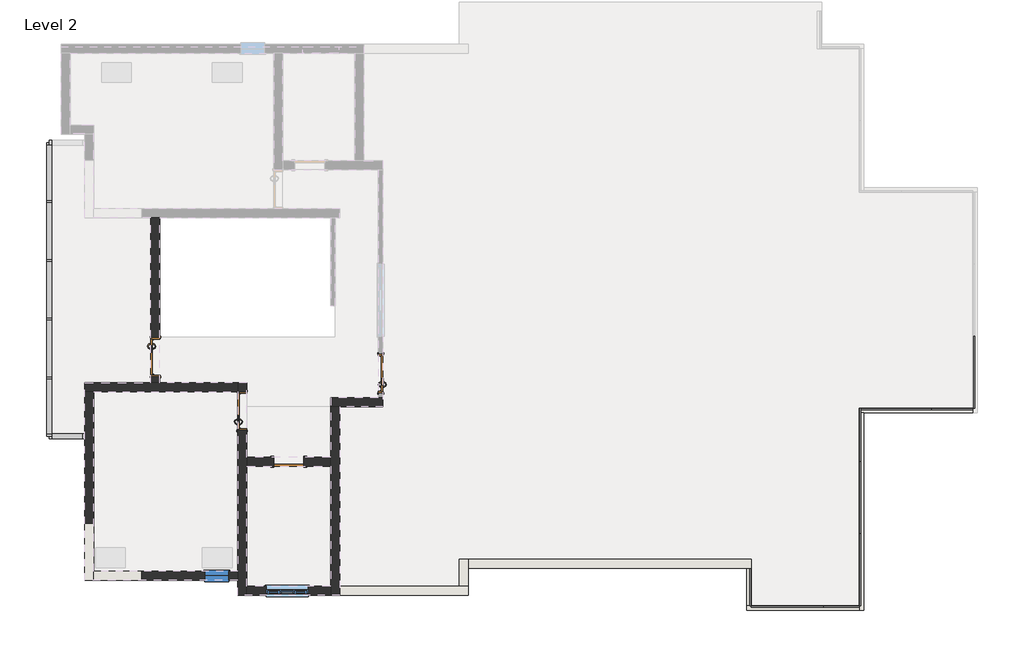
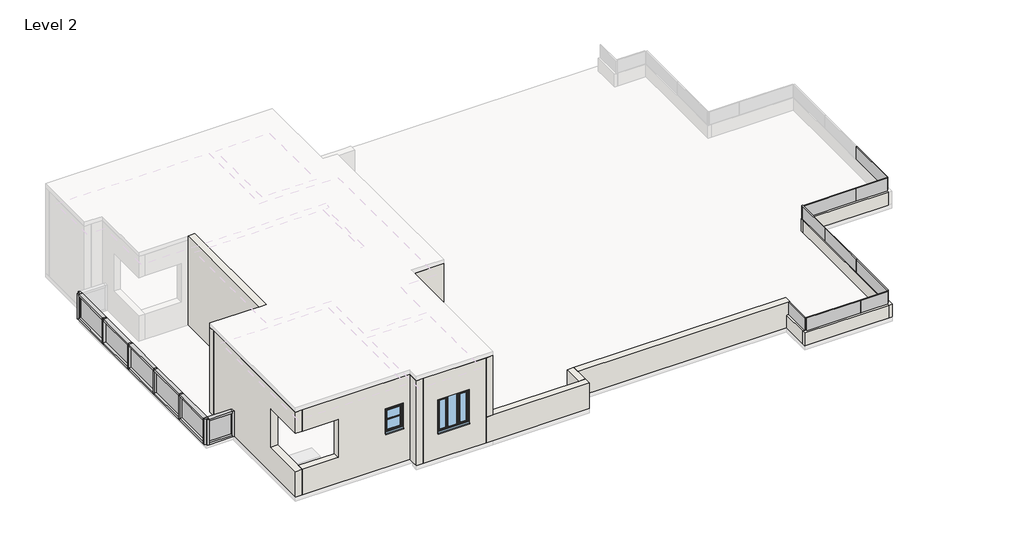
# One storey, part 1 of 2: 21 members, 16 walls, 15 plates, 4 doors, 2 windows.
"""IFC4 building model written with IfcOpenShell, lengths in millimetres."""

from ifc_helpers import new_model, si_unit, frame, origin, place, context, project, spatial, polyline, outline, extrude, faceted_brep, transform, mapped, element, save
from components import door_3dbecc4b, door_cca51ba5, door_181986ca, door_a1484949, member_429f6687, member_c646c215, member_7ec67256, member_73c23c35, member_410c6227, system_panel_glazed_cc3a876e, system_panel_glazed_f05af352, system_panel_glazed_b74e51ee, system_panel_glazed_cfd93610, system_panel_glazed_20ce4246, system_panel_glazed_26639370, system_panel_glazed_ff4fffb2, system_panel_glazed_c2969f63, windows_sgl_swept_head_window_2_x3_cc7253b0, window_63c4cdf6

model = new_model("IFC4")

# Units and contexts
model_context = context("Model", 3, world=origin())
ifc_project = project(units=[si_unit("LENGTHUNIT", "METRE", prefix="MILLI")], contexts=[model_context])

# Site, building, storey
site = spatial("IfcSite", under=ifc_project)
building = spatial("IfcBuilding", under=site)
storey = spatial("IfcBuildingStorey", under=building, Name="Level 2", Elevation=3200.4)

# Doors
placement = place(None, origin())
door_shape = door_3dbecc4b(model_context)
element("IfcDoor", 1, ObjectType="Doors_IntSgl_4 : Internal Door 3'3\"X7'", at=placement, inside=storey, context=model_context, shape_type="MappedRepresentation", body=[
    mapped(door_shape, transform((-3102.7378503, -1463.5864583, 3200.4), x_axis=(0.0, 1.0, 0.0), y_axis=(-1.0, 0.0, 0.0), z_axis=(0.0, 0.0, 1.0))),
])
door_2_shape = door_cca51ba5(model_context)
element("IfcDoor", 2, ObjectType="Doors_IntSgl_4 : Internal Door 3'3\"X7'", at=placement, inside=storey, context=model_context, shape_type="MappedRepresentation", body=[
    mapped(door_2_shape, transform((-5312.0457903, -91.9864583, 3200.4), x_axis=(0.0, -1.0, 0.0), y_axis=(1.0, 0.0, 0.0), z_axis=(0.0, 0.0, 1.0))),
])
door_3_shape = door_181986ca(model_context)
element("IfcDoor", 3, ObjectType="Doors_IntSgl_4 : Internal Door 3'3\"X7'", at=placement, inside=storey, context=model_context, shape_type="MappedRepresentation", body=[
    mapped(door_3_shape, transform((421.5121497, -511.0864583, 3200.4), x_axis=(0.0, 1.0, 0.0), y_axis=(-1.0, 0.0, 0.0), z_axis=(0.0, 0.0, 1.0))),
])
door_4_shape = door_a1484949(model_context)
element("IfcDoor", 4, ObjectType="Single-Flush : 2'6\"", at=placement, inside=storey, context=model_context, shape_type="MappedRepresentation", body=[
    mapped(door_4_shape, transform((-1921.6378503, -2759.0648645, 3200.4), x_axis=(-1.0, 0.0, 0.0), y_axis=(0.0, -1.0, 0.0), z_axis=(0.0, 0.0, 1.0))),
])

# Members
member_shape = member_429f6687(model_context)
element("IfcMember", 5, ObjectType="Rectangular Mullion : 2.5\" x 5\" rectangular", at=placement, inside=storey, context=model_context, shape_type="MappedRepresentation", body=[
    mapped(member_shape, transform((-7166.7378503, -2111.2864583, 4114.8), x_axis=(0.0, 0.0, 1.0), y_axis=(0.0, -1.0, 0.0), z_axis=(1.0, 0.0, 0.0))),
])
element("IfcMember", 6, ObjectType="Rectangular Mullion : 2.5\" x 5\" rectangular", at=placement, inside=storey, context=model_context, shape_type="MappedRepresentation", body=[
    mapped(member_shape, transform((-7954.1378503, -2111.2864583, 3200.4), x_axis=(0.0, 0.0, -1.0), y_axis=(0.0, -1.0, 0.0), z_axis=(-1.0, 0.0, 0.0))),
])
member_2_shape = member_c646c215(model_context)
element("IfcMember", 7, ObjectType="Rectangular Mullion : 2.5\" x 5\" rectangular", at=placement, inside=storey, context=model_context, shape_type="MappedRepresentation", body=[
    mapped(member_2_shape, transform((-8017.6378503, -2047.7864583, 4114.8), x_axis=(0.0, 0.0, 1.0), y_axis=(-1.0, 0.0, 0.0), z_axis=(0.0, -1.0, 0.0))),
])
element("IfcMember", 8, ObjectType="Rectangular Mullion : 2.5\" x 5\" rectangular", at=placement, inside=storey, context=model_context, shape_type="MappedRepresentation", body=[
    mapped(member_2_shape, transform((-8017.6378503, 3894.412299, 4114.8), x_axis=(0.0, 0.0, 1.0), y_axis=(-1.0, 0.0, 0.0), z_axis=(0.0, -1.0, 0.0))),
])
member_3_shape = member_7ec67256(model_context)
element("IfcMember", 9, ObjectType="Rectangular Mullion : 2.5\" x 5\" rectangular", at=placement, inside=storey, context=model_context, shape_type="MappedRepresentation", body=[
    mapped(member_3_shape, transform((-8017.6378503, 2400.9251098, 4114.8), x_axis=(0.0, 0.0, 1.0), y_axis=(-1.0, 0.0, 0.0), z_axis=(0.0, -1.0, 0.0))),
])
element("IfcMember", 10, ObjectType="Rectangular Mullion : 2.5\" x 5\" rectangular", at=placement, inside=storey, context=model_context, shape_type="MappedRepresentation", body=[
    mapped(member_3_shape, transform((-8017.6378503, 907.4379205, 4114.8), x_axis=(0.0, 0.0, 1.0), y_axis=(-1.0, 0.0, 0.0), z_axis=(0.0, -1.0, 0.0))),
])
element("IfcMember", 11, ObjectType="Rectangular Mullion : 2.5\" x 5\" rectangular", at=placement, inside=storey, context=model_context, shape_type="MappedRepresentation", body=[
    mapped(member_3_shape, transform((-8017.6378503, -586.0492687, 4114.8), x_axis=(0.0, 0.0, 1.0), y_axis=(-1.0, 0.0, 0.0), z_axis=(0.0, -1.0, 0.0))),
])
element("IfcMember", 12, ObjectType="Rectangular Mullion : 2.5\" x 5\" rectangular", at=placement, inside=storey, context=model_context, shape_type="MappedRepresentation", body=[
    mapped(member_2_shape, transform((-8017.6378503, 5292.6494886, 3200.4), x_axis=(0.0, 0.0, -1.0), y_axis=(-1.0, 0.0, 0.0), z_axis=(0.0, 1.0, 0.0))),
])
element("IfcMember", 13, ObjectType="Rectangular Mullion : 2.5\" x 5\" rectangular", at=placement, inside=storey, context=model_context, shape_type="MappedRepresentation", body=[
    mapped(member_2_shape, transform((-8017.6378503, -649.5492687, 3200.4), x_axis=(0.0, 0.0, -1.0), y_axis=(-1.0, 0.0, 0.0), z_axis=(0.0, 1.0, 0.0))),
])
element("IfcMember", 14, ObjectType="Rectangular Mullion : 2.5\" x 5\" rectangular", at=placement, inside=storey, context=model_context, shape_type="MappedRepresentation", body=[
    mapped(member_3_shape, transform((-8017.6378503, 3830.912299, 3200.4), x_axis=(0.0, 0.0, -1.0), y_axis=(-1.0, 0.0, 0.0), z_axis=(0.0, 1.0, 0.0))),
])
element("IfcMember", 15, ObjectType="Rectangular Mullion : 2.5\" x 5\" rectangular", at=placement, inside=storey, context=model_context, shape_type="MappedRepresentation", body=[
    mapped(member_3_shape, transform((-8017.6378503, 2337.4251098, 3200.4), x_axis=(0.0, 0.0, -1.0), y_axis=(-1.0, 0.0, 0.0), z_axis=(0.0, 1.0, 0.0))),
])
element("IfcMember", 16, ObjectType="Rectangular Mullion : 2.5\" x 5\" rectangular", at=placement, inside=storey, context=model_context, shape_type="MappedRepresentation", body=[
    mapped(member_3_shape, transform((-8017.6378503, 843.9379205, 3200.4), x_axis=(0.0, 0.0, -1.0), y_axis=(-1.0, 0.0, 0.0), z_axis=(0.0, 1.0, 0.0))),
])
member_4_shape = member_73c23c35(model_context)
element("IfcMember", 17, ObjectType="Rectangular Mullion : 2.5\" x 5\" rectangular", at=placement, inside=storey, context=model_context, shape_type="MappedRepresentation", body=[
    mapped(member_4_shape, transform((-8017.6378503, 5356.1494886, 3200.4), x_axis=(-1.0, 0.0, 0.0), y_axis=(0.0, 1.0, 0.0), z_axis=(0.0, 0.0, -1.0))),
])
element("IfcMember", 18, ObjectType="Rectangular Mullion : 2.5\" x 5\" rectangular", at=placement, inside=storey, context=model_context, shape_type="MappedRepresentation", body=[
    mapped(member_4_shape, transform((-8017.6378503, -2111.2864583, 3200.4), x_axis=(0.0, -1.0, 0.0), y_axis=(-1.0, 0.0, 0.0), z_axis=(0.0, 0.0, -1.0))),
])
element("IfcMember", 19, ObjectType="Rectangular Mullion : 2.5\" x 5\" rectangular", at=placement, inside=storey, context=model_context, shape_type="MappedRepresentation", body=[
    mapped(member_4_shape, transform((-7103.2378503, -2111.2864583, 3200.4), x_axis=(1.0, 0.0, 0.0), y_axis=(0.0, -1.0, 0.0), z_axis=(0.0, 0.0, -1.0))),
])
element("IfcMember", 20, ObjectType="Rectangular Mullion : 2.5\" x 5\" rectangular", at=placement, inside=storey, context=model_context, shape_type="MappedRepresentation", body=[
    mapped(member_4_shape, transform((-8017.6378503, 5356.1494886, 4114.8), x_axis=(0.0, 1.0, 0.0), y_axis=(-1.0, 0.0, 0.0), z_axis=(0.0, 0.0, 1.0))),
])
element("IfcMember", 21, ObjectType="Rectangular Mullion : 2.5\" x 5\" rectangular", at=placement, inside=storey, context=model_context, shape_type="MappedRepresentation", body=[
    mapped(member_4_shape, transform((-8017.6378503, -2111.2864583, 4114.8), x_axis=(-1.0, 0.0, 0.0), y_axis=(0.0, -1.0, 0.0), z_axis=(0.0, 0.0, 1.0))),
])
member_5_shape = member_410c6227(model_context)
element("IfcMember", 22, ObjectType="Rectangular Mullion : 2.5\" x 5\" rectangular", at=placement, inside=storey, context=model_context, shape_type="MappedRepresentation", body=[
    mapped(member_5_shape, transform((-8017.6378503, 3862.662299, 3200.4), x_axis=(0.0, -1.0, 0.0), y_axis=(-1.0, 0.0, 0.0), z_axis=(0.0, 0.0, -1.0))),
])
element("IfcMember", 23, ObjectType="Rectangular Mullion : 2.5\" x 5\" rectangular", at=placement, inside=storey, context=model_context, shape_type="MappedRepresentation", body=[
    mapped(member_5_shape, transform((-8017.6378503, 2369.1751098, 3200.4), x_axis=(0.0, -1.0, 0.0), y_axis=(-1.0, 0.0, 0.0), z_axis=(0.0, 0.0, -1.0))),
])
element("IfcMember", 24, ObjectType="Rectangular Mullion : 2.5\" x 5\" rectangular", at=placement, inside=storey, context=model_context, shape_type="MappedRepresentation", body=[
    mapped(member_5_shape, transform((-8017.6378503, 875.6879205, 3200.4), x_axis=(0.0, -1.0, 0.0), y_axis=(-1.0, 0.0, 0.0), z_axis=(0.0, 0.0, -1.0))),
])
element("IfcMember", 25, ObjectType="Rectangular Mullion : 2.5\" x 5\" rectangular", at=placement, inside=storey, context=model_context, shape_type="MappedRepresentation", body=[
    mapped(member_5_shape, transform((-8017.6378503, -617.7992687, 3200.4), x_axis=(0.0, -1.0, 0.0), y_axis=(-1.0, 0.0, 0.0), z_axis=(0.0, 0.0, -1.0))),
])

# Plates
system_panel_glazed_shape = system_panel_glazed_cc3a876e(model_context)
element("IfcPlate", 26, ObjectType="System Panel : Glazed", at=placement, inside=storey, context=model_context, shape_type="MappedRepresentation", body=[
    mapped(system_panel_glazed_shape, transform((9851.2621497, -5940.3364583, 3657.6), x_axis=(0.0, -1.0, 0.0), y_axis=(1.0, 0.0, 0.0), z_axis=(0.0, 0.0, 1.0))),
])
system_panel_glazed_2_shape = system_panel_glazed_f05af352(model_context)
element("IfcPlate", 27, ObjectType="System Panel : Glazed", at=placement, inside=storey, context=model_context, shape_type="MappedRepresentation", body=[
    mapped(system_panel_glazed_2_shape, transform((10765.6621499, -6416.5864583, 3657.6), x_axis=(1.0, 0.0, 0.0), y_axis=(0.0, 1.0, 0.0), z_axis=(0.0, 0.0, 1.0))),
])
element("IfcPlate", 28, ObjectType="System Panel : Glazed", at=placement, inside=storey, context=model_context, shape_type="MappedRepresentation", body=[
    mapped(system_panel_glazed_2_shape, transform((12594.4621497, -5502.1864581, 3657.6), x_axis=(0.0, 1.0, 0.0), y_axis=(-1.0, 0.0, 0.0), z_axis=(0.0, 0.0, 1.0))),
])
element("IfcPlate", 29, ObjectType="System Panel : Glazed", at=placement, inside=storey, context=model_context, shape_type="MappedRepresentation", body=[
    mapped(system_panel_glazed_2_shape, transform((12594.4621497, -3673.386458, 3657.6), x_axis=(0.0, 1.0, 0.0), y_axis=(-1.0, 0.0, 0.0), z_axis=(0.0, 0.0, 1.0))),
])
element("IfcPlate", 30, ObjectType="System Panel : Glazed", at=placement, inside=storey, context=model_context, shape_type="MappedRepresentation", body=[
    mapped(system_panel_glazed_2_shape, transform((13508.8621499, -1387.3864583, 3657.6), x_axis=(1.0, 0.0, 0.0), y_axis=(0.0, 1.0, 0.0), z_axis=(0.0, 0.0, 1.0))),
])
element("IfcPlate", 31, ObjectType="System Panel : Glazed", at=placement, inside=storey, context=model_context, shape_type="MappedRepresentation", body=[
    mapped(system_panel_glazed_2_shape, transform((15490.0621497, -472.9864581, 3657.6), x_axis=(0.0, 1.0, 0.0), y_axis=(-1.0, 0.0, 0.0), z_axis=(0.0, 0.0, 1.0))),
])
system_panel_glazed_3_shape = system_panel_glazed_b74e51ee(model_context)
element("IfcPlate", 32, ObjectType="System Panel : Glazed", at=placement, inside=storey, context=model_context, shape_type="MappedRepresentation", body=[
    mapped(system_panel_glazed_3_shape, transform((12137.2621499, -6416.5864583, 3657.6), x_axis=(1.0, 0.0, 0.0), y_axis=(0.0, 1.0, 0.0), z_axis=(0.0, 0.0, 1.0))),
])
system_panel_glazed_4_shape = system_panel_glazed_cfd93610(model_context)
element("IfcPlate", 33, ObjectType="System Panel : Glazed", at=placement, inside=storey, context=model_context, shape_type="MappedRepresentation", body=[
    mapped(system_panel_glazed_4_shape, transform((12594.4621497, -2073.1864581, 3657.6), x_axis=(0.0, 1.0, 0.0), y_axis=(-1.0, 0.0, 0.0), z_axis=(0.0, 0.0, 1.0))),
])
system_panel_glazed_5_shape = system_panel_glazed_20ce4246(model_context)
element("IfcPlate", 34, ObjectType="System Panel : Glazed", at=placement, inside=storey, context=model_context, shape_type="MappedRepresentation", body=[
    mapped(system_panel_glazed_5_shape, transform((14956.6621499, -1387.3864583, 3657.6), x_axis=(1.0, 0.0, 0.0), y_axis=(0.0, 1.0, 0.0), z_axis=(0.0, 0.0, 1.0))),
])
system_panel_glazed_6_shape = system_panel_glazed_26639370(model_context)
element("IfcPlate", 35, ObjectType="System Panel : Glazed", at=placement, inside=storey, context=model_context, shape_type="MappedRepresentation", body=[
    mapped(system_panel_glazed_6_shape, transform((-7560.4378503, -2111.2864583, 3263.9), x_axis=(1.0, 0.0, 0.0), y_axis=(0.0, 1.0, 0.0), z_axis=(0.0, 0.0, 1.0))),
])
system_panel_glazed_7_shape = system_panel_glazed_ff4fffb2(model_context)
element("IfcPlate", 36, ObjectType="System Panel : Glazed", at=placement, inside=storey, context=model_context, shape_type="MappedRepresentation", body=[
    mapped(system_panel_glazed_7_shape, transform((-8017.6378503, 4593.5308938, 3263.9), x_axis=(0.0, -1.0, 0.0), y_axis=(1.0, 0.0, 0.0), z_axis=(0.0, 0.0, 1.0))),
])
element("IfcPlate", 37, ObjectType="System Panel : Glazed", at=placement, inside=storey, context=model_context, shape_type="MappedRepresentation", body=[
    mapped(system_panel_glazed_7_shape, transform((-8017.6378503, -1348.6678635, 3263.9), x_axis=(0.0, -1.0, 0.0), y_axis=(1.0, 0.0, 0.0), z_axis=(0.0, 0.0, 1.0))),
])
system_panel_glazed_8_shape = system_panel_glazed_c2969f63(model_context)
element("IfcPlate", 38, ObjectType="System Panel : Glazed", at=placement, inside=storey, context=model_context, shape_type="MappedRepresentation", body=[
    mapped(system_panel_glazed_8_shape, transform((-8017.6378503, 3115.9187044, 3263.9), x_axis=(0.0, -1.0, 0.0), y_axis=(1.0, 0.0, 0.0), z_axis=(0.0, 0.0, 1.0))),
])
element("IfcPlate", 39, ObjectType="System Panel : Glazed", at=placement, inside=storey, context=model_context, shape_type="MappedRepresentation", body=[
    mapped(system_panel_glazed_8_shape, transform((-8017.6378503, 1622.4315152, 3263.9), x_axis=(0.0, -1.0, 0.0), y_axis=(1.0, 0.0, 0.0), z_axis=(0.0, 0.0, 1.0))),
])
element("IfcPlate", 40, ObjectType="System Panel : Glazed", at=placement, inside=storey, context=model_context, shape_type="MappedRepresentation", body=[
    mapped(system_panel_glazed_8_shape, transform((-8017.6378503, 128.9443259, 3263.9), x_axis=(0.0, -1.0, 0.0), y_axis=(1.0, 0.0, 0.0), z_axis=(0.0, 0.0, 1.0))),
])

# Walls
element("IfcWall", 41, ObjectType="Generic - 4.5\"", at=placement, inside=storey, context=model_context, shape_type="Brep", body=[
    faceted_brep([(15490.0621497, -1387.3864583, 3200.4), (12594.4621497, -1387.3864583, 3200.4), (12594.4621497, -1387.3864583, 3657.6), (15490.0621497, -1387.3864583, 3657.6), (15490.0621497, -1501.6864583, 3200.4), (15490.0621497, -1501.6864583, 3657.6), (12708.7621497, -1501.6864583, 3657.6), (12594.4621497, -1501.6864583, 3657.6), (12594.4621497, -1501.6864583, 3200.4), (12708.7621497, -1501.6864583, 3200.4)], [[[0, 1, 2, 3]], [[4, 5, 6, 7, 8, 9]], [[1, 0, 4, 9, 8]], [[3, 2, 7, 6, 5]], [[0, 3, 5, 4]], [[2, 1, 8, 7]]]),
])
element("IfcWall", 42, ObjectType="Generic - 4.5\"", at=placement, inside=storey, context=model_context, shape_type="Brep", body=[
    faceted_brep([(12594.4621497, -1501.6864583, 3200.4), (12594.4621497, -6416.5864583, 3200.4), (12594.4621497, -6530.8864583, 3200.4), (12594.4621497, -6530.8864583, 3657.6), (12594.4621497, -6416.5864583, 3657.6), (12594.4621497, -1501.6864583, 3657.6), (12708.7621497, -1501.6864583, 3200.4), (12708.7621497, -1501.6864583, 3657.6), (12708.7621497, -6530.8864583, 3657.6), (12708.7621497, -6530.8864583, 3200.4)], [[[0, 1, 2, 3, 4, 5]], [[6, 7, 8, 9]], [[2, 1, 0, 6, 9]], [[5, 4, 3, 8, 7]], [[0, 5, 7, 6]], [[3, 2, 9, 8]]]),
])
element("IfcWall", 43, ObjectType="Generic - 4.5\"", at=placement, inside=storey, context=model_context, shape_type="Brep", body=[
    faceted_brep([(12594.4621497, -6416.5864583, 3200.4), (9851.2621497, -6416.5864583, 3200.4), (9736.9621497, -6416.5864583, 3200.4), (9736.9621497, -6416.5864583, 3657.6), (9851.2621497, -6416.5864583, 3657.6), (12594.4621497, -6416.5864583, 3657.6), (12594.4621497, -6530.8864583, 3200.4), (12594.4621497, -6530.8864583, 3657.6), (9736.9621497, -6530.8864583, 3657.6), (9736.9621497, -6530.8864583, 3200.4)], [[[0, 1, 2, 3, 4, 5]], [[6, 7, 8, 9]], [[2, 1, 0, 6, 9]], [[5, 4, 3, 8, 7]], [[0, 5, 7, 6]], [[3, 2, 9, 8]]]),
])
element("IfcWall", 44, ObjectType="Generic - 4.5\"", at=placement, inside=storey, context=model_context, shape_type="SweptSolid", body=[
    extrude(outline(polyline([(9851.2621497, -5464.0864583), (9851.2621497, -6416.5864583), (9736.9621497, -6416.5864583), (9736.9621497, -5464.0864583), (9851.2621497, -5464.0864583)])), frame((0.0, 0.0, 3200.4), z_axis=(0.0, 0.0, 1.0), x_axis=(1.0, 0.0, 0.0)), (0.0, 0.0, 1.0), 457.2),
])
element("IfcWall", 45, ObjectType="Generic - 9\"", at=placement, inside=storey, context=model_context, shape_type="Brep", body=[
    faceted_brep([(-854.8378503, -6149.9648645, 3200.4), (2650.3621497, -6149.9648645, 3200.4), (2650.3621497, -6149.9648645, 4114.8), (-626.2378503, -6149.9648645, 4114.8), (-854.8378503, -6149.9648645, 4114.8), (-854.8378503, -5921.3648645, 3200.4), (-854.8378503, -5921.3648645, 4114.8), (-626.2378503, -5921.3648645, 4114.8), (2421.7621497, -5921.3648645, 4114.8), (2650.3621497, -5921.3648645, 4114.8), (2650.3621497, -5921.3648645, 3200.4), (2421.7621497, -5921.3648645, 3200.4), (-626.2378503, -5921.3648645, 3200.4)], [[[0, 1, 2, 3, 4]], [[5, 6, 7, 8, 9, 10, 11, 12]], [[1, 0, 5, 12, 11, 10]], [[4, 3, 2, 9, 8, 7, 6]], [[2, 1, 10, 9]], [[0, 4, 6, 5]]]),
])
element("IfcWall", 46, ObjectType="Generic - 9\"", at=placement, inside=storey, context=model_context, shape_type="Brep", body=[
    faceted_brep([(2650.3621497, -5921.3648645, 3200.4), (2650.3621497, -5464.0864583, 3200.4), (2650.3621497, -5235.4864583, 3200.4), (2650.3621497, -5235.4864583, 4114.8), (2650.3621497, -5464.0864583, 4114.8), (2650.3621497, -5921.3648645, 4114.8), (2421.7621497, -5921.3648645, 3200.4), (2421.7621497, -5921.3648645, 4114.8), (2421.7621497, -5235.4864583, 4114.8), (2421.7621497, -5235.4864583, 3200.4)], [[[0, 1, 2, 3, 4, 5]], [[6, 7, 8, 9]], [[2, 1, 0, 6, 9]], [[5, 4, 3, 8, 7]], [[0, 5, 7, 6]], [[3, 2, 9, 8]]]),
])
element("IfcWall", 47, ObjectType="Generic - 9\"", at=placement, inside=storey, context=model_context, shape_type="Brep", body=[
    faceted_brep([(2650.3621497, -5464.0864583, 3200.4), (9736.9621497, -5464.0864583, 3200.4), (9851.2621497, -5464.0864583, 3200.4), (9851.2621497, -5464.0864583, 3657.6), (9851.2621497, -5464.0864583, 4114.8), (2650.3621497, -5464.0864583, 4114.8), (2650.3621497, -5235.4864583, 3200.4), (2650.3621497, -5235.4864583, 4114.8), (9851.2621497, -5235.4864583, 4114.8), (9851.2621497, -5235.4864583, 3200.4)], [[[0, 1, 2, 3, 4, 5]], [[6, 7, 8, 9]], [[2, 1, 0, 6, 9]], [[5, 4, 8, 7]], [[0, 5, 7, 6]], [[4, 3, 2, 9, 8]]]),
])
element("IfcWall", 48, ObjectType="Generic - 9\"", at=placement, inside=storey, context=model_context, shape_type="SweptSolid", body=[
    extrude(outline(polyline([(-739.6864583, 6400.8), (3451.3135417, 6400.8), (3451.3135417, 3200.4), (403.3135417, 3200.4), (403.3135417, 5334.0), (-587.2864583, 5334.0), (-587.2864583, 3200.4), (-739.6864583, 3200.4), (-739.6864583, 6400.8)])), frame((-5426.3457903, 0.0, 0.0), z_axis=(1.0, 0.0, 0.0), x_axis=(0.0, 1.0, 0.0)), (0.0, 0.0, 1.0), 228.6),
])
element("IfcWall", 49, ObjectType="Generic - 9\"", at=placement, inside=storey, context=model_context, shape_type="Brep", body=[
    faceted_brep([(-3217.0378503, -739.6864583, 3200.4), (-5197.7457903, -739.6864583, 3200.4), (-5426.3457903, -739.6864583, 3200.4), (-7103.2378503, -739.6864583, 3200.4), (-7103.2378503, -739.6864583, 6248.4), (-5426.3457903, -739.6864583, 6248.4), (-3217.0378503, -739.6864583, 6248.4), (-3217.0378503, -968.2864583, 3200.4), (-3217.0378503, -968.2864583, 6248.4), (-6874.6378503, -968.2864583, 6248.4), (-7103.2378503, -968.2864583, 6248.4), (-7103.2378503, -968.2864583, 3200.4), (-6874.6378503, -968.2864583, 3200.4)], [[[0, 1, 2, 3, 4, 5, 6]], [[7, 8, 9, 10, 11, 12]], [[3, 2, 1, 0, 7, 12, 11]], [[4, 3, 11, 10]], [[0, 6, 8, 7]], [[6, 5, 4, 10, 9, 8]]]),
])
element("IfcWall", 50, ObjectType="Generic - 9\"", at=placement, inside=storey, context=model_context, shape_type="Brep", body=[
    faceted_brep([(-7103.2378503, -968.2864583, 3200.4), (-7103.2378503, -5768.8864583, 3200.4), (-7103.2378503, -5768.8864583, 4114.8), (-7103.2378503, -4317.8481466, 4114.8), (-7103.2378503, -4317.8481466, 5486.4), (-7103.2378503, -5768.8864583, 5486.4), (-7103.2378503, -5768.8864583, 6248.4), (-7103.2378503, -968.2864583, 6248.4), (-6874.6378503, -5768.8864583, 3200.4), (-6874.6378503, -5540.2864583, 3200.4), (-6874.6378503, -968.2864583, 3200.4), (-6874.6378503, -968.2864583, 6248.4), (-6874.6378503, -5540.2864583, 6248.4), (-6874.6378503, -5768.8864583, 6248.4), (-6874.6378503, -5768.8864583, 5486.4), (-6874.6378503, -5540.2864583, 5486.4), (-6874.6378503, -4317.8481466, 5486.4), (-6874.6378503, -4317.8481466, 4114.8), (-6874.6378503, -5540.2864583, 4114.8), (-6874.6378503, -5768.8864583, 4114.8)], [[[0, 1, 2, 3, 4, 5, 6, 7]], [[8, 9, 10, 11, 12, 13, 14, 15, 16, 17, 18, 19]], [[1, 0, 10, 9, 8]], [[0, 7, 11, 10]], [[4, 16, 15, 14, 5]], [[17, 3, 2, 19, 18]], [[16, 4, 3, 17]], [[1, 8, 19, 2]], [[13, 6, 5, 14]], [[7, 6, 13, 12, 11]]]),
])
element("IfcWall", 51, ObjectType="Generic - 9\"", at=placement, inside=storey, context=model_context, shape_type="SweptSolid", body=[
    extrude(outline(polyline([(3200.4, -6874.6378503), (3200.4, -3217.0378503), (6248.4, -3217.0378503), (6248.4, -6874.6378503), (5486.4, -6874.6378503), (5486.4, -5658.7498785), (4114.8, -5658.7498785), (4114.8, -6874.6378503), (3200.4, -6874.6378503)]), holes=[polyline([(5310.4, -3445.6378503), (4396.0, -3445.6378503), (4396.0, -4055.2378503), (5310.4, -4055.2378503), (5310.4, -3445.6378503)])]), frame((0.0, -5768.8864583, 0.0), z_axis=(0.0, 1.0, 0.0), x_axis=(0.0, 0.0, 1.0)), (0.0, 0.0, 1.0), 228.6),
])
element("IfcWall", 52, ObjectType="Generic - 9\"", at=placement, inside=storey, context=model_context, shape_type="Brep", body=[
    faceted_brep([(-2988.4378503, -739.6864583, 3200.4), (-2988.4378503, -739.6864583, 6248.4), (-2988.4378503, -2644.7648645, 6248.4), (-2988.4378503, -2873.3648645, 6248.4), (-2988.4378503, -5921.3648645, 6248.4), (-2988.4378503, -6149.9648645, 6248.4), (-2988.4378503, -6149.9648645, 3200.4), (-2988.4378503, -5921.3648645, 3200.4), (-2988.4378503, -2873.3648645, 3200.4), (-2988.4378503, -2644.7648645, 3200.4), (-2988.4378503, -1958.8864583, 3200.4), (-2988.4378503, -1958.8864583, 5334.0), (-2988.4378503, -968.2864583, 5334.0), (-2988.4378503, -968.2864583, 3200.4), (-3217.0378503, -739.6864583, 6248.4), (-3217.0378503, -739.6864583, 3200.4), (-3217.0378503, -968.2864583, 3200.4), (-3217.0378503, -968.2864583, 5334.0), (-3217.0378503, -1958.8864583, 5334.0), (-3217.0378503, -1958.8864583, 3200.4), (-3217.0378503, -5540.2864583, 3200.4), (-3217.0378503, -5768.8864583, 3200.4), (-3217.0378503, -6149.9648645, 3200.4), (-3217.0378503, -6149.9648645, 6248.4), (-3217.0378503, -5768.8864583, 6248.4), (-3217.0378503, -5540.2864583, 6248.4), (-3217.0378503, -968.2864583, 6248.4)], [[[0, 1, 2, 3, 4, 5, 6, 7, 8, 9, 10, 11, 12, 13]], [[14, 15, 16, 17, 18, 19, 20, 21, 22, 23, 24, 25, 26]], [[15, 0, 13, 16]], [[6, 22, 21, 20, 19, 10, 9, 8, 7]], [[1, 0, 15, 14]], [[6, 5, 23, 22]], [[12, 17, 16, 13]], [[17, 12, 11, 18]], [[18, 11, 10, 19]], [[23, 5, 4, 3, 2, 1, 14, 26, 25, 24]]]),
])
element("IfcWall", 53, ObjectType="Generic - 9\"", at=placement, inside=storey, context=model_context, shape_type="SweptSolid", body=[
    extrude(outline(polyline([(3200.4, -2988.4378503), (3200.4, -2302.6378503), (5232.4, -2302.6378503), (5232.4, -1540.6378503), (3200.4, -1540.6378503), (3200.4, -854.8378503), (6248.4, -854.8378503), (6248.4, -2988.4378503), (3200.4, -2988.4378503)])), frame((0.0, -2873.3648645, 0.0), z_axis=(0.0, 1.0, 0.0), x_axis=(0.0, 0.0, 1.0)), (0.0, 0.0, 1.0), 228.6),
])
element("IfcWall", 54, ObjectType="Generic - 9\"", at=placement, inside=storey, context=model_context, shape_type="Brep", body=[
    faceted_brep([(-854.8378503, -1349.2864583, 3200.4), (-626.2378503, -1349.2864583, 3200.4), (478.6621497, -1349.2864583, 3200.4), (478.6621497, -1349.2864583, 6248.4), (-626.2378503, -1349.2864583, 6248.4), (-854.8378503, -1349.2864583, 6248.4), (-854.8378503, -1120.6864583, 3200.4), (-854.8378503, -1120.6864583, 6248.4), (364.3621497, -1120.6864583, 6248.4), (478.6621497, -1120.6864583, 6248.4), (478.6621497, -1120.6864583, 3200.4), (364.3621497, -1120.6864583, 3200.4)], [[[0, 1, 2, 3, 4, 5]], [[6, 7, 8, 9, 10, 11]], [[2, 1, 0, 6, 11, 10]], [[0, 5, 7, 6]], [[3, 2, 10, 9]], [[5, 4, 3, 9, 8, 7]]]),
])
element("IfcWall", 55, ObjectType="Generic - 9\"", at=placement, inside=storey, context=model_context, shape_type="Brep", body=[
    faceted_brep([(-854.8378503, -1349.2864583, 3200.4), (-854.8378503, -2644.7648645, 3200.4), (-854.8378503, -2873.3648645, 3200.4), (-854.8378503, -5921.3648645, 3200.4), (-854.8378503, -5921.3648645, 4114.8), (-854.8378503, -6149.9648645, 4114.8), (-854.8378503, -6149.9648645, 6248.4), (-854.8378503, -5921.3648645, 6248.4), (-854.8378503, -2873.3648645, 6248.4), (-854.8378503, -2644.7648645, 6248.4), (-854.8378503, -1349.2864583, 6248.4), (-626.2378503, -1349.2864583, 3200.4), (-626.2378503, -1349.2864583, 6248.4), (-626.2378503, -6149.9648645, 6248.4), (-626.2378503, -6149.9648645, 4114.8), (-626.2378503, -5921.3648645, 4114.8), (-626.2378503, -5921.3648645, 3200.4)], [[[0, 1, 2, 3, 4, 5, 6, 7, 8, 9, 10]], [[11, 12, 13, 14, 15, 16]], [[3, 2, 1, 0, 11, 16]], [[0, 10, 12, 11]], [[14, 5, 4, 15]], [[4, 3, 16, 15]], [[6, 5, 14, 13]], [[10, 9, 8, 7, 6, 13, 12]]]),
])
element("IfcWall", 56, ObjectType="Generic - 9\"", at=placement, inside=storey, context=model_context, shape_type="Brep", body=[
    faceted_brep([(-854.8378503, -5921.3648645, 3200.4), (-2988.4378503, -5921.3648645, 3200.4), (-2988.4378503, -5921.3648645, 6248.4), (-854.8378503, -5921.3648645, 6248.4), (-854.8378503, -5921.3648645, 4114.8), (-1426.3378503, -5921.3648645, 5310.4), (-2493.1378503, -5921.3648645, 5310.4), (-2493.1378503, -5921.3648645, 4091.2), (-1426.3378503, -5921.3648645, 4091.2), (-854.8378503, -6149.9648645, 3200.4), (-854.8378503, -6149.9648645, 4114.8), (-854.8378503, -6149.9648645, 6248.4), (-2988.4378503, -6149.9648645, 6248.4), (-2988.4378503, -6149.9648645, 3200.4), (-1426.3378503, -6149.9648645, 5310.4), (-1426.3378503, -6149.9648645, 4091.2), (-2493.1378503, -6149.9648645, 4091.2), (-2493.1378503, -6149.9648645, 5310.4)], [[[0, 1, 2, 3, 4], [5, 6, 7, 8]], [[9, 10, 11, 12, 13], [14, 15, 16, 17]], [[1, 0, 9, 13]], [[0, 4, 3, 11, 10, 9]], [[2, 1, 13, 12]], [[15, 14, 5, 8]], [[16, 15, 8, 7]], [[17, 16, 7, 6]], [[14, 17, 6, 5]], [[3, 2, 12, 11]]]),
])

# Windows
windows_sgl_swept_head_window_2_x3_shape = windows_sgl_swept_head_window_2_x3_cc7253b0(model_context)
element("IfcWindow", 57, ObjectType="Windows_Sgl_Swept_Head : Window 2'X3'", at=placement, inside=storey, context=model_context, shape_type="MappedRepresentation", body=[
    mapped(windows_sgl_swept_head_window_2_x3_shape, transform((-3750.4378503, -5646.1298904, 3200.4), x_axis=(-1.0, 0.0, 0.0), y_axis=(0.0, -1.0, 0.0), z_axis=(0.0, 0.0, 1.0))),
])
window_shape = window_63c4cdf6(model_context)
element("IfcWindow", 58, ObjectType="Windows_Tpl_Plain : Window 3'6\"X4'", at=placement, inside=storey, context=model_context, shape_type="MappedRepresentation", body=[
    mapped(window_shape, transform((-2412.5378503, -6027.2082967, 3200.4), x_axis=(-1.0, 0.0, 0.0), y_axis=(0.0, -1.0, 0.0), z_axis=(0.0, 0.0, 1.0))),
])

save(model, "model.ifc")

# Revit data of these elements
# Type "Doors_IntSgl_4 : Internal Door 3'3\"X7'"
#   Type Mark = "13"
#   Type Comments = "Internal Single"
#   Operation = "SingleSwingRight"
#   Construction Type Id = "SGL"
#   Manufacturer = "Revit"
#   Keynote = "L20"
#   Description = "Internal Single Door"
#   Analytic Construction = "Large single-glazed windows"
#   Visual Light Transmittance = 0.9
#   VisionPanel Width = 0' - 7.28346"
#   VisionPanel Depth = 0' - 7.28346"
#   UnderCut = 0' - 0.31496"
#   Tolerance = 0' - 0.07874"
#   Thickness = 0' - 1.49606"
#   Structural Tolerance = 0' - 0.31496"
#   StopDepth = 0' - 1.25984"
#   Stop Thickness = 0' - 0.74803"
#   Stile Shutting = 0' - 6.10236"
#   Stile Top Rail = 0' - 9.84252"
#   Stile Intermediate/Frieze = 0' - 3.93701"
#   Solar Heat Gain Coefficient = 0.86
#   Rough Width = 3' - 3"
#   Rough Height = 7' - 0"
#   Heat Transfer Coefficient (U) = 0.979472 BTU/(h·ft²·°F)
#   Handle Z Distance = 3' - 3.37008"
#   Handle X Distance = 0' - 2.95276"
#   Handle Length = 1' - 1.77953"
#   Frame Thickness = 0' - 1.25984"
#   Door Panel Width = 2' - 11.69291"
#   Door Panel Thickness = 0' - 1.49606"
#   Door Panel Offset = 0' - 0"
#   Height = 7' - 0"
#   Width = 3' - 3"
#   Door Panel Height = 6' - 10.0315"
#   Architrave Setback = 0' - 0.19685"
#   Vis - Ironmongery = yes
#   Define Thermal Properties by = 1
#   Material Ironmongery = Door - Handle
#   Material Glass = Door - Glazing
#   Material Frame = Door - Frame/Mullion
#   Material Door = Door - Panel
#   Material Beading = Door - Panel
#   Material Architrave = Door - Architrave
#   Handle Style = element 386699
#   Function = (empty or 0)
#   Wall Closure = (empty or 0)
# Type "Single-Flush : 2'6\""
#   Type Mark = "14"
#   Construction Type Id = "MDOOR"
#   Assembly Code = "C1020"
#   Analytic Construction = "Metal"
#   Rough Width = 2' - 6"
#   Rough Height = 7' - 0"
#   Thickness = 0' - 2"
#   Heat Transfer Coefficient (U) = 0.651978 BTU/(h·ft²·°F)
#   Height = 6' - 8"
#   Trim Projection Ext = 0' - 1"
#   Trim Projection Int = 0' - 1"
#   Trim Width = 0' - 3"
#   Width = 2' - 6"
#   Define Thermal Properties by = 1
#   Door Material = Door - Panel
#   Frame Material = Door - Frame
#   Visual Light Transmittance = 0
#   Solar Heat Gain Coefficient = 0
#   Function = (empty or 0)
#   Wall Closure = (empty or 0)
# Type "Rectangular Mullion : 2.5\" x 5\" rectangular"
#   built-in parameter 1007304 = 0.416667 (stored number, unit not read)
#   built-in parameter 1007301 = 0.104167 (stored number, unit not read)
#   built-in parameter 1007300 = 0.104167 (stored number, unit not read)
# Type "System Panel : Glazed"
#   Construction Type Id = "GSP4R"
#   Analytic Construction = "1/8 in Pilkington single glazing"
#   Visual Light Transmittance = 0.9
#   Solar Heat Gain Coefficient = 0.86
#   Heat Transfer Coefficient (U) = 1.18115 BTU/(h·ft²·°F)
#   Define Thermal Properties by = 1
# Type "Generic - 4.5\""
#   Assembly Code = "B2010"
#   Layers, outside or top first: 0' - 4 1/2" no material (function 1)
# Type "Generic - 9\""
#   Assembly Code = "B2010"
#   Layers, outside or top first: 0' - 9" no material (function 1)
# Type "Windows_Sgl_Swept_Head : Window 2'X3'"
#   Type Mark = "31"
#   Operation = "SinglePanel"
#   Construction Type Id = "SGL"
#   Manufacturer = "Revit"
#   Keynote = "L10"
#   Analytic Construction = "Large single-glazed windows"
#   Wrap Layers (Ext) from Ext = 0' - 4.03543"
#   Wrap Layers (Int) from Ext = 0' - 6.98819"
#   Window Board Projection = 0' - 0.98425"
#   Window Board Extension = 0' - 0.98425"
#   Visual Light Transmittance = 0.9
#   Solar Heat Gain Coefficient = 0.86
#   Rough Width = 2' - 0"
#   Rough Height = 3' - 0"
#   Radius - Swept Head = 2' - 11.81102"
#   Height = 3' - 0"
#   Width = 2' - 0"
#   Heat Transfer Coefficient (U) = 0.979472 BTU/(h·ft²·°F)
#   Glazing Thickness = 0' - 0.94488"
#   FrameOffset - External = 0' - 1.9685"
#   Frame Depth = 0' - 2.55906"
#   Default Head Height = 6' - 11.07087"
#   Cill Depth = 0' - 3.44488"
#   Cavity Closer Width = 0' - 1.9685"
#   Cavity Closer Offset from Ext = 0' - 4.03543"
#   Cavity Closer Depth = 0' - 3.34646"
#   Vis - Cavity Closers = yes
#   Define Thermal Properties by = 1
#   Material Trim = Window Frame
#   Material Glass = Glass
#   Material Frame = Window Frame
#   Wall Closure = (empty or 0)
# Type "Windows_Tpl_Plain : Window 3'6\"X4'"
#   Type Mark = "33"
#   Operation = "TriplePanelVertical"
#   Construction Type Id = "GSP4R"
#   Manufacturer = "Revit"
#   Keynote = "L10"
#   Analytic Construction = "1/8 in Pilkington single glazing"
#   Wrap Layers (Ext) from Ext = 0' - 4.03543"
#   Wrap Layers (Int) from Ext = 0' - 6.98819"
#   Window Board Projection = 0' - 0.98425"
#   Window Board Extension = 0' - 0.98425"
#   Visual Light Transmittance = 0.9
#   Solar Heat Gain Coefficient = 0.78
#   Rough Width = 3' - 6"
#   Rough Height = 4' - 0"
#   Height = 4' - 0"
#   Width = 3' - 6"
#   Heat Transfer Coefficient (U) = 0.6496 BTU/(h·ft²·°F)
#   Glazing Thickness = 0' - 0.94488"
#   FrameOffset - External = 0' - 1.9685"
#   Frame Depth = 0' - 2.55906"
#   Default Head Height = 6' - 11.07087"
#   Cill Depth = 0' - 3.44488"
#   Cavity Closer Width = 0' - 1.9685"
#   Cavity Closer Offset from Ext = 0' - 4.03543"
#   Cavity Closer Depth = 0' - 3.34646"
#   Vis - Cavity Closers = yes
#   Define Thermal Properties by = 1
#   Material Trim = Window Frame
#   Material Glass = Glass
#   Material Frame = Window Frame
#   Wall Closure = (empty or 0)
# Elements 1, 2, 3 (IfcDoor, "Doors_IntSgl_4 : Internal Door 3'3\"X7'")
#   Phase Created = New Construction
#   Materials on its faces: "Door - Panel", "Door - Architrave", "Door - Handle", "Door - Frame/Mullion", "Door - Glazing"
# Element 4 (IfcDoor, "Single-Flush : 2'6\"")
#   Phase Created = New Construction
#   Materials on its faces: "Door - Frame", "Door - Panel"
# Elements 5, 6, 7, 8, 9, 10, 11, 12, 13, 14, 15, 16, 17, 18, 19, 20, 21, 22, 23, 24, 25 (IfcMember, "Rectangular Mullion : 2.5\" x 5\" rectangular")
#   Phase Created = New Construction
#   Materials on its faces: "Aluminum"
# Elements 26, 27, 28, 29, 30, 31, 32, 33, 34, 35, 36, 37, 38, 39, 40 (IfcPlate, "System Panel : Glazed")
#   Phase Created = New Construction
#   Materials on its faces: "Glass"
# Elements 41, 42, 43 (IfcWall, "Generic - 4.5\"")
#   Top Offset = 0' - 0"
#   Base Offset = 0' - 0"
#   Unconnected Height = 1' - 6"
#   wall height = 1' - 6"
#   Phase Created = New Construction
#   Base Constraint = Level 2
#   Materials on its faces: "Default Wall", "Beige Colour"
# Element 44 (IfcWall, "Generic - 4.5\"")
#   Top Offset = 0' - 0"
#   Base Offset = 0' - 0"
#   Unconnected Height = 1' - 6"
#   wall height = 1' - 6"
#   Phase Created = New Construction
#   Base Constraint = Level 2
#   Materials on its faces: "Default Wall"
# Elements 45, 46, 47 (IfcWall, "Generic - 9\"")
#   Top Offset = 0' - 0"
#   Base Offset = 0' - 0"
#   Unconnected Height = 3' - 0"
#   wall height = 3' - 0"
#   Phase Created = New Construction
#   Base Constraint = Level 2
#   Materials on its faces: "Default Wall", "Beige Colour"
# Element 48 (IfcWall, "Generic - 9\"")
#   Top Offset = 0' - 0"
#   Base Offset = 0' - 0"
#   Unconnected Height = 10' - 6"
#   wall height = 10' - 6"
#   Phase Created = New Construction
#   Base Constraint = Level 2
#   Top Constraint = Level 3
#   Materials on its faces: "Default Wall", "Beige Colour"
# Elements 49, 50, 51, 52, 54, 55, 56 (IfcWall, "Generic - 9\"")
#   Top Offset = 0' - 0"
#   Base Offset = 0' - 0"
#   wall height = 10' - 0"
#   Phase Created = New Construction
#   Base Constraint = Level 2
#   Top Constraint = Level 3
#   Materials on its faces: "Default Wall", "Beige Colour"
# Element 53 (IfcWall, "Generic - 9\"")
#   Top Offset = 0' - 0"
#   Base Offset = 0' - 0"
#   wall height = 10' - 0"
#   Phase Created = New Construction
#   Base Constraint = Level 2
#   Top Constraint = Level 3
#   Materials on its faces: "Default Wall"
# Element 57 (IfcWindow, "Windows_Sgl_Swept_Head : Window 2'X3'")
#   Mark = "14"
#   Phase Created = New Construction
#   Materials on its faces: "Window Frame", "Glass"
# Element 58 (IfcWindow, "Windows_Tpl_Plain : Window 3'6\"X4'")
#   Mark = "11"
#   Phase Created = New Construction
#   Materials on its faces: "Window Frame", "Glass"
# Materials
#   "Door - Handle": colour RGB 247 247 247, transparency 0
#   "Door - Glazing": colour RGB 0 0 255, transparency 0.75
#   "Door - Frame/Mullion": class "Wood", colour RGB 212 179 113, transparency 0
#   "Door - Panel": class "Wood", colour RGB 210 159 95, transparency 0, Cost = 0
#   "Door - Architrave": class "Wood", colour RGB 212 179 113, transparency 0
#   "Door - Frame": colour RGB 118 70 51, transparency 0, Cost = 0
#   "Window Frame": colour RGB 249 249 249, transparency 0
#   "Glass": class "Glass", colour RGB 0 128 192, transparency 0.75, Description = "Soda Lime Glass", Cost = 0
#   "Aluminum": class "Metal", colour RGB 247 247 247, transparency 0, Description = "Aluminum 6061", Cost = 0
#   "Default Wall": colour RGB 128 128 128, transparency 0, Cost = 0
#   "Beige Colour": class "Generic", colour RGB 120 120 120, transparency 0, Cost = 0
